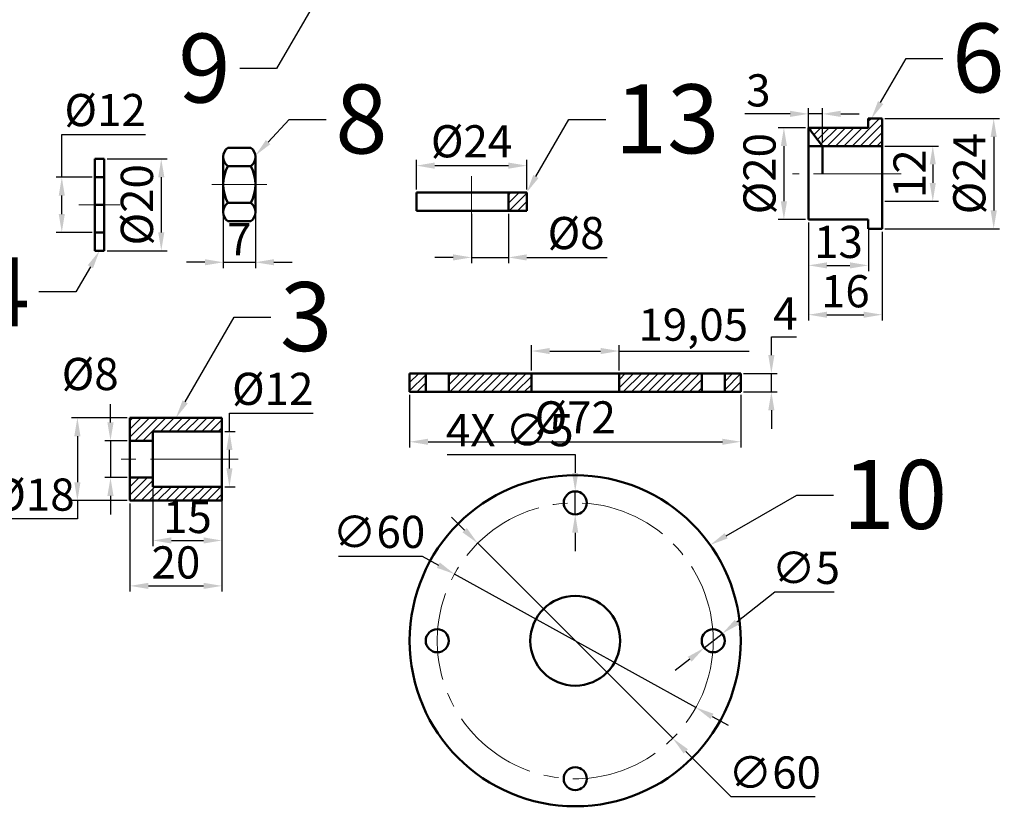
# Model space of a CAD drawing. Units: millimetres. Extents: x 123 to 731, y 468 to 864.
# Tile 3 of 5: x 328 to 542, y 604 to 775. Entities that reach past the tile are written whole.
import ezdxf
from ezdxf import colors
from ezdxf.entities.mleader import LeaderData, LeaderLine
from ezdxf.math import Vec2, Vec3

# ---------------------------------------------------------------- set-up
doc = ezdxf.new("R2010")
doc.units = ezdxf.units.MM
doc.linetypes.add('CENTER2', pattern=[28.575, 19.05, -3.175, 3.175, -3.175])
for name, color, linetype, lineweight in [('M-CNTR', 1, 'CENTER2', 18), ('M-DIMS', 2, 'Continuous', 25), ('M-HATC', 8, 'Continuous', 18), ('M-OUTL', 7, 'Continuous', 50), ('M-TEXT', 3, 'Continuous', 25)]:
    doc.layers.add(name, color=color, linetype=linetype, lineweight=lineweight)
doc.styles.get("Standard").update_dxf_attribs({"font": 'arial.ttf'})
doc.dimstyles.new('ISO-25', dxfattribs={"dimtxt": 7, "dimasz": 4, "dimexe": 1.25, "dimexo": 0.625, "dimtad": 1, "dimtoh": 1, "dimtxsty": 'Standard', "dimcen": 2.5, "dimadec": 0, "dimazin": 0, "dimtfac": 1, "dimtmove": 0, "dimatfit": 3, "dimfxl": 1, "dimarcsym": 0})

# ---------------------------------------------------------------- blocks, each defined once
blk = doc.blocks.new('*D38')
at = {"layer": 'Defpoints', "color": 0, "transparency": 16777216}
for p in [(372.22, 733.55), (379.22, 733.55), (379.22, 722.64)]:
    blk.add_point(p, dxfattribs=at)
at = {"layer": 'M-DIMS', "color": 0, "lineweight": -2, "transparency": 16777216}
for p, q in [((372.22, 732.92), (372.22, 721.39)), ((379.22, 732.92), (379.22, 721.39)), ((368.22, 722.64), (364.22, 722.64)), ((372.22, 722.64), (379.22, 722.64)), ((383.22, 722.64), (387.22, 722.64))]:
    blk.add_line(p, q, dxfattribs=at)
at = {"layer": 'M-DIMS', "color": 0, "transparency": 16777216}
for points in [[(368.22, 723.31), (368.22, 721.98), (372.22, 722.64)], [(383.22, 723.31), (383.22, 721.98), (379.22, 722.64)]]:
    blk.add_solid(points, dxfattribs=at)
at = {"layer": 'M-DIMS', "color": 0, "transparency": 16777216, "insert": (375.72, 726.77), "char_height": 7, "attachment_point": 5}
blk.add_mtext('7', dxfattribs=at)
blk = doc.blocks.new('*U39')
at = {"layer": 'M-CNTR', "color": 0, "transparency": 16777216}
blk.add_line((6, 0), (-6, 0), dxfattribs=at)
blk = doc.blocks.new('*U41')
at = {"layer": 'M-CNTR', "color": 0, "transparency": 16777216}
blk.add_line((4.5, 0), (-4.5, 0), dxfattribs=at)
blk = doc.blocks.new('*D43')
at = {"layer": 'Defpoints', "color": 0, "transparency": 16777216}
for p in [(344.32, 741.14), (337.11, 729.14), (344.32, 729.14)]:
    blk.add_point(p, dxfattribs=at)
at = {"layer": 'M-DIMS', "color": 0, "lineweight": -2, "transparency": 16777216}
for p, q in [((337.11, 741.14), (337.11, 750.44)), ((337.11, 750.44), (355.3, 750.44)), ((343.7, 741.14), (335.86, 741.14)), ((337.11, 733.14), (337.11, 737.14)), ((343.7, 729.14), (335.86, 729.14))]:
    blk.add_line(p, q, dxfattribs=at)
at = {"layer": 'M-DIMS', "color": 0, "transparency": 16777216}
for points in [[(336.44, 737.14), (337.77, 737.14), (337.11, 741.14)], [(336.44, 733.14), (337.77, 733.14), (337.11, 729.14)]]:
    blk.add_solid(points, dxfattribs=at)
at = {"layer": 'M-DIMS', "color": 0, "transparency": 16777216, "insert": (346.52, 754.84), "char_height": 7, "attachment_point": 5}
blk.add_mtext('%%C12', dxfattribs=at)
blk = doc.blocks.new('*D44')
at = {"layer": 'Defpoints', "color": 0, "transparency": 16777216}
for p in [(346.32, 745.14), (346.32, 725.14), (358.74, 725.14)]:
    blk.add_point(p, dxfattribs=at)
at = {"layer": 'M-DIMS', "color": 0, "lineweight": -2, "transparency": 16777216}
for p, q in [((346.95, 745.14), (359.99, 745.14)), ((358.74, 741.14), (358.74, 729.14)), ((346.95, 725.14), (359.99, 725.14))]:
    blk.add_line(p, q, dxfattribs=at)
at = {"layer": 'M-DIMS', "color": 0, "transparency": 16777216}
for points in [[(358.08, 741.14), (359.41, 741.14), (358.74, 745.14)], [(358.08, 729.14), (359.41, 729.14), (358.74, 725.14)]]:
    blk.add_solid(points, dxfattribs=at)
at = {"layer": 'M-DIMS', "color": 0, "transparency": 16777216, "insert": (354.35, 735.14), "char_height": 7, "attachment_point": 5, "rotation": 90}
blk.add_mtext('%%C20', dxfattribs=at)
blk = doc.blocks.new('*U45')
at = {"layer": 'M-CNTR', "color": 0, "transparency": 16777216}
blk.add_line((0, -5.5), (0, 5.5), dxfattribs=at)
blk = doc.blocks.new('*D47')
at = {"layer": 'Defpoints', "color": 0, "transparency": 16777216}
for p in [(438.21, 743.66), (414.21, 737.84), (438.21, 737.84)]:
    blk.add_point(p, dxfattribs=at)
at = {"layer": 'M-DIMS', "color": 0, "lineweight": -2, "transparency": 16777216}
for p, q in [((414.21, 738.46), (414.21, 744.91)), ((418.21, 743.66), (434.21, 743.66)), ((438.21, 738.46), (438.21, 744.91))]:
    blk.add_line(p, q, dxfattribs=at)
at = {"layer": 'M-DIMS', "color": 0, "transparency": 16777216}
for points in [[(418.21, 744.33), (418.21, 742.99), (414.21, 743.66)], [(434.21, 744.33), (434.21, 742.99), (438.21, 743.66)]]:
    blk.add_solid(points, dxfattribs=at)
at = {"layer": 'M-DIMS', "color": 0, "transparency": 16777216, "insert": (426.21, 748.05), "char_height": 7, "attachment_point": 5}
blk.add_mtext('%%C24', dxfattribs=at)
blk = doc.blocks.new('*D48')
at = {"layer": 'Defpoints', "color": 0, "transparency": 16777216}
for p in [(426.21, 733.84), (434.21, 733.84), (434.21, 723.7)]:
    blk.add_point(p, dxfattribs=at)
at = {"layer": 'M-DIMS', "color": 0, "lineweight": -2, "transparency": 16777216}
for p, q in [((426.21, 733.21), (426.21, 722.45)), ((434.21, 733.21), (434.21, 722.45)), ((422.21, 723.7), (418.21, 723.7)), ((426.21, 723.7), (434.21, 723.7)), ((438.21, 723.7), (455.68, 723.7))]:
    blk.add_line(p, q, dxfattribs=at)
at = {"layer": 'M-DIMS', "color": 0, "transparency": 16777216}
for points in [[(422.21, 724.36), (422.21, 723.03), (426.21, 723.7)], [(438.21, 724.36), (438.21, 723.03), (434.21, 723.7)]]:
    blk.add_solid(points, dxfattribs=at)
at = {"layer": 'M-DIMS', "color": 0, "transparency": 16777216, "insert": (448.94, 728.09), "char_height": 7, "attachment_point": 5}
blk.add_mtext('%%C8', dxfattribs=at)
blk = doc.blocks.new('*U54')
at = {"layer": 'M-CNTR', "color": 0, "transparency": 16777216}
blk.add_line((13.65, 0), (-10, 0), dxfattribs=at)
blk = doc.blocks.new('*D55')
at = {"layer": 'Defpoints', "color": 0, "transparency": 16777216}
for p in [(499.49, 751.91), (494.13, 731.91), (499.49, 731.91)]:
    blk.add_point(p, dxfattribs=at)
at = {"layer": 'M-DIMS', "color": 0, "lineweight": -2, "transparency": 16777216}
for p, q in [((498.86, 751.91), (492.88, 751.91)), ((494.13, 747.91), (494.13, 735.91)), ((498.86, 731.91), (492.88, 731.91))]:
    blk.add_line(p, q, dxfattribs=at)
at = {"layer": 'M-DIMS', "color": 0, "transparency": 16777216}
for points in [[(493.46, 747.91), (494.8, 747.91), (494.13, 751.91)], [(493.46, 735.91), (494.8, 735.91), (494.13, 731.91)]]:
    blk.add_solid(points, dxfattribs=at)
at = {"layer": 'M-DIMS', "color": 0, "transparency": 16777216, "insert": (489.73, 741.91), "char_height": 7, "attachment_point": 5, "rotation": 90}
blk.add_mtext('%%C20', dxfattribs=at)
blk = doc.blocks.new('*D56')
at = {"layer": 'Defpoints', "color": 0, "transparency": 16777216}
for p in [(502.49, 754.92), (499.49, 747.91), (502.49, 747.91)]:
    blk.add_point(p, dxfattribs=at)
at = {"layer": 'M-DIMS', "color": 0, "lineweight": -2, "transparency": 16777216}
for p, q in [((499.49, 748.54), (499.49, 756.17)), ((502.49, 748.54), (502.49, 756.17)), ((495.49, 754.92), (485.65, 754.92)), ((502.49, 754.92), (499.49, 754.92)), ((506.49, 754.92), (510.49, 754.92))]:
    blk.add_line(p, q, dxfattribs=at)
at = {"layer": 'M-DIMS', "color": 0, "transparency": 16777216}
for points in [[(495.49, 755.59), (495.49, 754.25), (499.49, 754.92)], [(506.49, 755.59), (506.49, 754.25), (502.49, 754.92)]]:
    blk.add_solid(points, dxfattribs=at)
at = {"layer": 'M-DIMS', "color": 0, "transparency": 16777216, "insert": (488.57, 759.12), "char_height": 7, "attachment_point": 5}
blk.add_mtext('3', dxfattribs=at)
blk = doc.blocks.new('*D57')
at = {"layer": 'Defpoints', "color": 0, "transparency": 16777216}
for p in [(515.49, 747.91), (515.49, 735.91), (526.5, 735.91)]:
    blk.add_point(p, dxfattribs=at)
at = {"layer": 'M-DIMS', "color": 0, "lineweight": -2, "transparency": 16777216}
for p, q in [((516.11, 747.91), (527.75, 747.91)), ((526.5, 743.91), (526.5, 739.91)), ((516.11, 735.91), (527.75, 735.91))]:
    blk.add_line(p, q, dxfattribs=at)
at = {"layer": 'M-DIMS', "color": 0, "transparency": 16777216}
for points in [[(525.83, 743.91), (527.17, 743.91), (526.5, 747.91)], [(525.83, 739.91), (527.17, 739.91), (526.5, 735.91)]]:
    blk.add_solid(points, dxfattribs=at)
at = {"layer": 'M-DIMS', "color": 0, "transparency": 16777216, "insert": (522.36, 741.91), "char_height": 7, "attachment_point": 5, "rotation": 90}
blk.add_mtext('12', dxfattribs=at)
blk = doc.blocks.new('*D58')
at = {"layer": 'Defpoints', "color": 0, "transparency": 16777216}
for p in [(515.49, 753.91), (515.49, 729.91), (539.75, 729.91)]:
    blk.add_point(p, dxfattribs=at)
at = {"layer": 'M-DIMS', "color": 0, "lineweight": -2, "transparency": 16777216}
for p, q in [((516.11, 753.91), (541, 753.91)), ((539.75, 749.91), (539.75, 733.91)), ((516.11, 729.91), (541, 729.91))]:
    blk.add_line(p, q, dxfattribs=at)
at = {"layer": 'M-DIMS', "color": 0, "transparency": 16777216}
for points in [[(539.08, 749.91), (540.42, 749.91), (539.75, 753.91)], [(539.08, 733.91), (540.42, 733.91), (539.75, 729.91)]]:
    blk.add_solid(points, dxfattribs=at)
at = {"layer": 'M-DIMS', "color": 0, "transparency": 16777216, "insert": (535.36, 741.91), "char_height": 7, "attachment_point": 5, "rotation": 90}
blk.add_mtext('%%C24', dxfattribs=at)
blk = doc.blocks.new('*D59')
at = {"layer": 'Defpoints', "color": 0, "transparency": 16777216}
for p in [(499.49, 731.91), (512.49, 731.91), (512.49, 721.97)]:
    blk.add_point(p, dxfattribs=at)
at = {"layer": 'M-DIMS', "color": 0, "lineweight": -2, "transparency": 16777216}
for p, q in [((499.49, 731.29), (499.49, 720.72)), ((512.49, 731.29), (512.49, 720.72)), ((503.49, 721.97), (508.49, 721.97))]:
    blk.add_line(p, q, dxfattribs=at)
at = {"layer": 'M-DIMS', "color": 0, "transparency": 16777216}
for points in [[(503.49, 722.63), (503.49, 721.3), (499.49, 721.97)], [(508.49, 722.63), (508.49, 721.3), (512.49, 721.97)]]:
    blk.add_solid(points, dxfattribs=at)
at = {"layer": 'M-DIMS', "color": 0, "transparency": 16777216, "insert": (505.99, 726.17), "char_height": 7, "attachment_point": 5}
blk.add_mtext('13', dxfattribs=at)
blk = doc.blocks.new('*D60')
at = {"layer": 'Defpoints', "color": 0, "transparency": 16777216}
for p in [(499.49, 731.91), (515.49, 729.91), (515.49, 711.24)]:
    blk.add_point(p, dxfattribs=at)
at = {"layer": 'M-DIMS', "color": 0, "lineweight": -2, "transparency": 16777216}
for p, q in [((499.49, 731.29), (499.49, 709.99)), ((515.49, 729.29), (515.49, 709.99)), ((503.49, 711.24), (511.49, 711.24))]:
    blk.add_line(p, q, dxfattribs=at)
at = {"layer": 'M-DIMS', "color": 0, "transparency": 16777216}
for points in [[(503.49, 711.9), (503.49, 710.57), (499.49, 711.24)], [(511.49, 711.9), (511.49, 710.57), (515.49, 711.24)]]:
    blk.add_solid(points, dxfattribs=at)
at = {"layer": 'M-DIMS', "color": 0, "transparency": 16777216, "insert": (507.49, 715.44), "char_height": 7, "attachment_point": 5}
blk.add_mtext('16', dxfattribs=at)
blk = doc.blocks.new('*U70')
at = {"layer": 'M-CNTR', "color": 0, "transparency": 16777216}
blk.add_line((13.5, 0), (-13.5, 0), dxfattribs=at)
blk = doc.blocks.new('*D72')
at = {"layer": 'Defpoints', "color": 0, "transparency": 16777216}
for p in [(351.93, 683.82), (347.7, 675.82), (351.93, 675.82)]:
    blk.add_point(p, dxfattribs=at)
at = {"layer": 'M-DIMS', "color": 0, "lineweight": -2, "transparency": 16777216}
for p, q in [((347.7, 687.82), (347.7, 691.82)), ((351.31, 683.82), (346.45, 683.82)), ((347.7, 683.82), (347.7, 675.82)), ((351.31, 675.82), (346.45, 675.82)), ((347.7, 671.82), (347.7, 667.82))]:
    blk.add_line(p, q, dxfattribs=at)
at = {"layer": 'M-DIMS', "color": 0, "transparency": 16777216}
for points in [[(347.03, 687.82), (348.37, 687.82), (347.7, 683.82)], [(347.03, 671.82), (348.37, 671.82), (347.7, 675.82)]]:
    blk.add_solid(points, dxfattribs=at)
at = {"layer": 'M-DIMS', "color": 0, "transparency": 16777216, "insert": (343.28, 697.44), "char_height": 7, "attachment_point": 5}
blk.add_mtext('%%C8', dxfattribs=at)
blk = doc.blocks.new('*D73')
at = {"layer": 'Defpoints', "color": 0, "transparency": 16777216}
for p in [(351.93, 688.82), (340.5, 670.82), (351.93, 670.82)]:
    blk.add_point(p, dxfattribs=at)
at = {"layer": 'M-DIMS', "color": 0, "lineweight": -2, "transparency": 16777216}
for p, q in [((351.31, 688.82), (339.25, 688.82)), ((340.5, 684.82), (340.5, 674.82)), ((351.31, 670.82), (339.25, 670.82)), ((340.5, 670.82), (340.5, 666.82)), ((340.5, 666.82), (322.22, 666.82))]:
    blk.add_line(p, q, dxfattribs=at)
at = {"layer": 'M-DIMS', "color": 0, "transparency": 16777216}
for points in [[(339.83, 684.82), (341.17, 684.82), (340.5, 688.82)], [(339.83, 674.82), (341.17, 674.82), (340.5, 670.82)]]:
    blk.add_solid(points, dxfattribs=at)
at = {"layer": 'M-DIMS', "color": 0, "transparency": 16777216, "insert": (331.05, 671.21), "char_height": 7, "attachment_point": 5}
blk.add_mtext('%%C18', dxfattribs=at)
blk = doc.blocks.new('*D74')
at = {"layer": 'Defpoints', "color": 0, "transparency": 16777216}
for p in [(356.93, 673.82), (371.93, 673.82), (371.93, 662.14)]:
    blk.add_point(p, dxfattribs=at)
at = {"layer": 'M-DIMS', "color": 0, "lineweight": -2, "transparency": 16777216}
for p, q in [((356.93, 673.19), (356.93, 660.89)), ((371.93, 673.19), (371.93, 660.89)), ((360.93, 662.14), (367.93, 662.14))]:
    blk.add_line(p, q, dxfattribs=at)
at = {"layer": 'M-DIMS', "color": 0, "transparency": 16777216}
for points in [[(360.93, 662.81), (360.93, 661.48), (356.93, 662.14)], [(367.93, 662.81), (367.93, 661.48), (371.93, 662.14)]]:
    blk.add_solid(points, dxfattribs=at)
at = {"layer": 'M-DIMS', "color": 0, "transparency": 16777216, "insert": (364.43, 666.34), "char_height": 7, "attachment_point": 5}
blk.add_mtext('15', dxfattribs=at)
blk = doc.blocks.new('*D75')
at = {"layer": 'Defpoints', "color": 0, "transparency": 16777216}
for p in [(351.93, 670.82), (371.93, 670.82), (371.93, 652.26)]:
    blk.add_point(p, dxfattribs=at)
at = {"layer": 'M-DIMS', "color": 0, "lineweight": -2, "transparency": 16777216}
for p, q in [((351.93, 670.19), (351.93, 651.01)), ((371.93, 670.19), (371.93, 651.01)), ((355.93, 652.26), (367.93, 652.26))]:
    blk.add_line(p, q, dxfattribs=at)
at = {"layer": 'M-DIMS', "color": 0, "transparency": 16777216}
for points in [[(355.93, 652.93), (355.93, 651.6), (351.93, 652.26)], [(367.93, 652.93), (367.93, 651.6), (371.93, 652.26)]]:
    blk.add_solid(points, dxfattribs=at)
at = {"layer": 'M-DIMS', "color": 0, "transparency": 16777216, "insert": (361.93, 656.46), "char_height": 7, "attachment_point": 5}
blk.add_mtext('20', dxfattribs=at)
blk = doc.blocks.new('*D76')
at = {"layer": 'Defpoints', "color": 0, "transparency": 16777216}
for p in [(371.93, 685.82), (371.93, 673.82), (373.56, 673.82)]:
    blk.add_point(p, dxfattribs=at)
at = {"layer": 'M-DIMS', "color": 0, "lineweight": -2, "transparency": 16777216}
for p, q in [((373.56, 685.82), (373.56, 689.82)), ((373.56, 689.82), (391.76, 689.82)), ((372.56, 685.82), (374.81, 685.82)), ((373.56, 677.82), (373.56, 681.82)), ((372.56, 673.82), (374.81, 673.82))]:
    blk.add_line(p, q, dxfattribs=at)
at = {"layer": 'M-DIMS', "color": 0, "transparency": 16777216}
for points in [[(372.9, 681.82), (374.23, 681.82), (373.56, 685.82)], [(372.9, 677.82), (374.23, 677.82), (373.56, 673.82)]]:
    blk.add_solid(points, dxfattribs=at)
at = {"layer": 'M-DIMS', "color": 0, "transparency": 16777216, "insert": (382.97, 694.21), "char_height": 7, "attachment_point": 5}
blk.add_mtext('%%C12', dxfattribs=at)
blk = doc.blocks.new('*D77')
at = {"layer": 'Defpoints', "color": 0, "transparency": 16777216}
for p in [(412.75, 694.45), (484.75, 694.45), (484.75, 683.61)]:
    blk.add_point(p, dxfattribs=at)
at = {"layer": 'M-DIMS', "color": 0, "lineweight": -2, "transparency": 16777216}
for p, q in [((412.75, 693.83), (412.75, 682.36)), ((484.75, 693.83), (484.75, 682.36)), ((416.75, 683.61), (480.75, 683.61))]:
    blk.add_line(p, q, dxfattribs=at)
at = {"layer": 'M-DIMS', "color": 0, "transparency": 16777216}
for points in [[(416.75, 684.27), (416.75, 682.94), (412.75, 683.61)], [(480.75, 684.27), (480.75, 682.94), (484.75, 683.61)]]:
    blk.add_solid(points, dxfattribs=at)
at = {"layer": 'M-DIMS', "color": 0, "transparency": 16777216, "insert": (448.75, 688), "char_height": 7, "attachment_point": 5}
blk.add_mtext('%%C72', dxfattribs=at)
blk = doc.blocks.new('*D78')
at = {"layer": 'Defpoints', "color": 0, "transparency": 16777216}
for p in [(458.28, 703.34), (439.23, 698.45), (458.28, 698.45)]:
    blk.add_point(p, dxfattribs=at)
at = {"layer": 'M-DIMS', "color": 0, "lineweight": -2, "transparency": 16777216}
for p, q in [((439.23, 699.08), (439.23, 704.59)), ((458.28, 699.08), (458.28, 704.59)), ((443.23, 703.34), (454.28, 703.34)), ((458.28, 703.34), (486.54, 703.34))]:
    blk.add_line(p, q, dxfattribs=at)
at = {"layer": 'M-DIMS', "color": 0, "transparency": 16777216}
for points in [[(443.23, 704.01), (443.23, 702.67), (439.23, 703.34)], [(454.28, 704.01), (454.28, 702.67), (458.28, 703.34)]]:
    blk.add_solid(points, dxfattribs=at)
at = {"layer": 'M-DIMS', "color": 0, "transparency": 16777216, "insert": (474.41, 708.17), "char_height": 7, "attachment_point": 5}
blk.add_mtext('19,05', dxfattribs=at)
blk = doc.blocks.new('*D79')
at = {"layer": 'Defpoints', "color": 0, "transparency": 16777216}
for p in [(480.71, 641.87), (476.79, 638.78)]:
    blk.add_point(p, dxfattribs=at)
at = {"layer": 'M-DIMS', "color": 0, "lineweight": -2, "transparency": 16777216}
for p, q in [((492.15, 650.88), (483.86, 644.35)), ((505.03, 650.88), (492.15, 650.88)), ((476.79, 638.78), (480.71, 641.87)), ((473.65, 636.3), (470.5, 633.83))]:
    blk.add_line(p, q, dxfattribs=at)
at = {"layer": 'M-DIMS', "color": 0, "transparency": 16777216}
for points in [[(483.44, 644.87), (484.27, 643.82), (480.71, 641.87)], [(473.23, 636.83), (474.06, 635.78), (476.79, 638.78)]]:
    blk.add_solid(points, dxfattribs=at)
at = {"layer": 'M-DIMS', "color": 0, "transparency": 16777216, "insert": (498.9, 655.27), "char_height": 7, "attachment_point": 5}
blk.add_mtext('∅5', dxfattribs=at)
blk = doc.blocks.new('*D80')
at = {"layer": 'Defpoints', "color": 0, "transparency": 16777216}
for p in [(422.49, 654.83), (475.01, 625.81)]:
    blk.add_point(p, dxfattribs=at)
at = {"layer": 'M-DIMS', "color": 0, "lineweight": -2, "transparency": 16777216}
for p, q in [((397.25, 658.7), (415.49, 658.7)), ((415.49, 658.7), (418.99, 656.77)), ((475.01, 625.81), (422.49, 654.83)), ((478.51, 623.88), (482.01, 621.95))]:
    blk.add_line(p, q, dxfattribs=at)
at = {"layer": 'M-DIMS', "color": 0, "transparency": 16777216}
for points in [[(419.31, 657.35), (418.67, 656.19), (422.49, 654.83)], [(478.83, 624.46), (478.19, 623.3), (475.01, 625.81)]]:
    blk.add_solid(points, dxfattribs=at)
at = {"layer": 'M-DIMS', "color": 0, "transparency": 16777216, "insert": (406.06, 663.1), "char_height": 7, "attachment_point": 5}
blk.add_mtext('∅60', dxfattribs=at)
blk = doc.blocks.new('HEX-NUT')
for p, q in [((6.02, 16), (1.02, 16)), ((1.02, 12), (6.02, 12)), ((1.02, 4), (6.02, 4)), ((1.02, 0), (6.02, 0))]:
    blk.add_line(p, q)
for centre, radius, start, end in [((2.47, 14), 2.47, 125.9888, 234.0112), ((4.57, 14), 2.47, 305.9888, 54.0112), ((8.52, 8), 8.5, 151.9275, 208.0725), ((-1.48, 8), 8.5, 331.9275, 28.0725), ((2.52, 2), 2.5, 126.8697, 233.1303), ((4.52, 2), 2.5, 306.8697, 53.1303)]:
    blk.add_arc(centre, radius, start, end)
blk = doc.blocks.new('*D94')
at = {"layer": 'Defpoints', "color": 0, "transparency": 16777216}
for p in [(484.75, 698.45), (491.4, 698.45), (484.75, 694.45)]:
    blk.add_point(p, dxfattribs=at)
at = {"layer": 'M-DIMS', "color": 0, "lineweight": -2, "transparency": 16777216}
for p, q in [((491.4, 702.45), (491.4, 706.45)), ((491.4, 706.45), (496.87, 706.45)), ((485.38, 698.45), (492.65, 698.45)), ((491.4, 694.45), (491.4, 698.45)), ((485.38, 694.45), (492.65, 694.45)), ((491.4, 690.45), (491.4, 686.45))]:
    blk.add_line(p, q, dxfattribs=at)
at = {"layer": 'M-DIMS', "color": 0, "transparency": 16777216}
for points in [[(490.73, 702.45), (492.07, 702.45), (491.4, 698.45)], [(490.73, 690.45), (492.07, 690.45), (491.4, 694.45)]]:
    blk.add_solid(points, dxfattribs=at)
at = {"layer": 'M-DIMS', "color": 0, "transparency": 16777216, "insert": (494.45, 710.58), "char_height": 7, "attachment_point": 5}
blk.add_mtext('4', dxfattribs=at)
blk = doc.blocks.new('*D96')
at = {"layer": 'Defpoints', "color": 0, "transparency": 16777216}
for p in [(427.54, 661.54), (469.96, 619.11)]:
    blk.add_point(p, dxfattribs=at)
at = {"layer": 'M-DIMS', "color": 0, "lineweight": -2, "transparency": 16777216}
for p, q in [((424.71, 664.37), (421.88, 667.2)), ((427.54, 661.54), (469.96, 619.11)), ((482.69, 606.38), (472.79, 616.28)), ((500.93, 606.38), (482.69, 606.38))]:
    blk.add_line(p, q, dxfattribs=at)
at = {"layer": 'M-DIMS', "color": 0, "transparency": 16777216}
for points in [[(425.18, 664.84), (424.24, 663.9), (427.54, 661.54)], [(473.26, 616.75), (472.32, 615.81), (469.96, 619.11)]]:
    blk.add_solid(points, dxfattribs=at)
at = {"layer": 'M-DIMS', "color": 0, "transparency": 16777216, "insert": (492.12, 610.77), "char_height": 7, "attachment_point": 5}
blk.add_mtext('∅60', dxfattribs=at)
blk = doc.blocks.new('*D97')
at = {"layer": 'Defpoints', "color": 0, "transparency": 16777216}
for p in [(448.75, 672.82), (448.75, 667.82)]:
    blk.add_point(p, dxfattribs=at)
at = {"layer": 'M-DIMS', "color": 0, "lineweight": -2, "transparency": 16777216}
for p, q in [((420.91, 680.82), (448.75, 680.82)), ((448.75, 680.82), (448.75, 676.82)), ((448.75, 667.82), (448.75, 672.82)), ((448.75, 663.82), (448.76, 659.82))]:
    blk.add_line(p, q, dxfattribs=at)
at = {"layer": 'M-DIMS', "color": 0, "transparency": 16777216}
for points in [[(449.41, 676.83), (448.08, 676.82), (448.75, 672.82)], [(449.42, 663.83), (448.09, 663.82), (448.75, 667.82)]]:
    blk.add_solid(points, dxfattribs=at)
at = {"layer": 'M-DIMS', "color": 0, "transparency": 16777216, "insert": (434.52, 685.22), "char_height": 7, "attachment_point": 5}
blk.add_mtext('4X ∅5', dxfattribs=at)

msp = doc.modelspace()

# ---------------------------------------------------------------- hatches: boundary and pattern name
at = {"layer": 'M-HATC'}
h = msp.add_hatch(dxfattribs=at)
h.set_pattern_fill('ANSI31', color=256, scale=0.4)
h.set_pattern_definition([(45, (-32.4287, 0), (-0.8980256, 0.8980256), [])])
h.paths.add_polyline_path([(499.4872, 751.9133), (502.4872, 747.9133), (515.4872, 747.9133), (515.4872, 753.9133), (512.4872, 753.9133), (512.4872, 751.9133)])
h = msp.add_hatch(dxfattribs=at)
h.set_pattern_fill('ANSI31', color=256, scale=0.4)
h.set_pattern_definition([(45, (-30.5264, 6.709), (-0.8980256, 0.8980256), [])])
h.paths.add_polyline_path([(434.2097, 733.837), (438.2097, 733.837), (438.2097, 737.837), (434.2097, 737.837)])
h = msp.add_hatch(dxfattribs=at)
h.set_pattern_fill('ANSI31', color=256, scale=0.4)
h.set_pattern_definition([(45, (-31.5995, 122.8167), (-0.8980256, 0.8980256), [])])
h.paths.add_polyline_path([(416.251, 698.4517), (412.751, 698.4517), (412.751, 694.4517), (416.251, 694.4517)])
h.paths.add_polyline_path([(439.226, 694.4517), (439.226, 698.4517), (421.251, 698.4517), (421.251, 694.4517)])
h.paths.add_polyline_path([(476.251, 694.4517), (476.251, 698.4517), (458.276, 698.4517), (458.276, 694.4517)])
h.paths.add_polyline_path([(481.251, 694.4517), (484.751, 694.4517), (484.751, 698.4517), (481.251, 698.4517)])
h = msp.add_hatch(dxfattribs=at)
h.set_pattern_fill('ANSI31', color=256, scale=0.4)
h.set_pattern_definition([(45, (-13.901, 8.0257), (-0.8980256, 0.8980256), [])])
h.paths.add_polyline_path([(351.9314, 683.8159), (356.9314, 683.8159), (356.9314, 685.8159), (371.9314, 685.8159), (371.9314, 688.8159), (351.9314, 688.8159)])
h.paths.add_polyline_path([(371.9314, 670.8159), (371.9314, 673.8159), (356.9314, 673.8159), (356.9314, 675.8159), (351.9314, 675.8159), (351.9314, 670.8159)])

# ---------------------------------------------------------------- linework, layer by layer
at = {"layer": 'M-CNTR'}
msp.add_circle((448.751, 640.3248), 30, dxfattribs=at)
at = {"layer": 'M-OUTL'}
for p, q in [((515.4872, 753.9133), (512.4872, 753.9133)), ((512.4872, 753.9133), (512.4872, 751.9133)), ((515.4872, 729.9133), (515.4872, 753.9133)), ((499.4872, 751.9133), (499.4872, 731.9133)), ((512.4872, 751.9133), (499.4872, 751.9133)), ((502.4872, 747.9133), (499.4872, 751.9133)), ((499.4872, 747.9133), (502.4872, 747.9133)), ((502.4872, 747.9133), (502.4872, 741.9133)), ((502.4872, 747.9133), (515.4872, 747.9133)), ((344.3205, 745.1393), (344.3205, 725.1393)), ((346.3205, 745.1393), (344.3205, 745.1393)), ((346.3205, 725.1393), (346.3205, 745.1393)), ((372.2169, 745.8609), (372.2169, 733.5485)), ((379.2169, 733.5485), (379.2169, 745.8609)), ((344.3205, 741.1393), (346.3205, 741.1393)), ((438.2097, 737.837), (414.2097, 737.837)), ((414.2097, 737.837), (414.2097, 733.837)), ((434.2097, 737.837), (434.2097, 733.837)), ((438.2097, 733.837), (438.2097, 737.837)), ((344.3205, 735.1393), (346.3205, 735.1393)), ((414.2097, 733.837), (438.2097, 733.837)), ((499.4872, 731.9133), (512.4872, 731.9133)), ((512.4872, 731.9133), (512.4872, 729.9133)), ((344.3205, 729.1393), (346.3205, 729.1393)), ((512.4872, 729.9133), (515.4872, 729.9133)), ((344.3205, 725.1393), (346.3205, 725.1393)), ((484.751, 698.4517), (412.751, 698.4517)), ((412.751, 698.4517), (412.751, 694.4517)), ((416.251, 694.4517), (416.251, 698.4517)), ((421.251, 694.4517), (421.251, 698.4517)), ((439.226, 698.4517), (439.226, 694.4517)), ((458.276, 698.4517), (458.276, 694.4517)), ((476.251, 694.4517), (476.251, 698.4517)), ((481.251, 694.4517), (481.251, 698.4517)), ((484.751, 694.4517), (484.751, 698.4517)), ((412.751, 694.4517), (484.751, 694.4517)), ((351.9314, 688.8159), (351.9314, 670.8159)), ((371.9314, 688.8159), (351.9314, 688.8159)), ((371.9314, 670.8159), (371.9314, 688.8159)), ((371.9314, 685.8159), (356.9314, 685.8159)), ((356.9314, 685.8159), (356.9314, 673.8159)), ((351.9314, 683.8159), (356.9314, 683.8159)), ((351.9314, 675.8159), (356.9314, 675.8159)), ((356.9314, 673.8159), (371.9314, 673.8159)), ((351.9314, 670.8159), (371.9314, 670.8159))]:
    msp.add_line(p, q, dxfattribs=at)
for centre, radius in [((448.751, 640.3248), 36), ((448.751, 670.3248), 2.5), ((448.751, 640.3248), 9.7625), ((418.751, 640.3248), 2.5), ((478.751, 640.3248), 2.5), ((448.751, 610.3248), 2.5)]:
    msp.add_circle(centre, radius, dxfattribs=at)

# ---------------------------------------------------------------- block references
at = {"layer": 'M-CNTR'}
for name, p in [('*U45', (426.2097, 735.837)), ('*U54', (505.9872, 741.9133)), ('*U39', (375.7169, 739.5526)), ('*U41', (345.3205, 735.1393)), ('*U70', (361.9314, 679.8159))]:
    msp.add_blockref(name, p, dxfattribs=at)
at = {"layer": 'M-OUTL'}
msp.add_blockref('HEX-NUT', (372.198, 731.553), dxfattribs=at)

# ---------------------------------------------------------------- dimensions: what is measured, and where the dimension line sits
at = {"layer": 'M-DIMS'}
dim = msp.add_linear_dim(base=(502.4872, 754.9192), p1=(499.4872, 747.9133), p2=(502.4872, 747.9133), dimstyle='ISO-25', override={"dimclrd": 0, "dimclre": 0, "dimclrt": 0}, dxfattribs=at)
dim.commit()
dim.dimension.update_dxf_attribs({"geometry": '*D56', "text_midpoint": (488.5702, 754.9192), "dimtype": 160})
for base, p1, p2, override, picture, middle in [((337.1058, 729.1393), (344.3205, 741.1393), (344.3205, 729.1393), {"dimclrd": 0, "dimclre": 0, "dimclrt": 0}, '*D43', (346.5166, 750.4444)), ((347.7005, 675.8159), (351.9314, 683.8159), (351.9314, 675.8159), {"dimclrd": 0, "dimclre": 0, "dimclrt": 0, "dimtmove": 2}, '*D72', (343.2759, 697.4433)), ((373.5627, 673.8159), (371.9314, 685.8159), (371.9314, 673.8159), {"dimclrd": 0, "dimclre": 0, "dimclrt": 0}, '*D76', (382.9736, 689.8159))]:
    dim = msp.add_linear_dim(base=base, p1=p1, p2=p2, angle=90, text='%%C<>', dimstyle='ISO-25', override=override, dxfattribs=at)
    dim.commit()
    dim.dimension.update_dxf_attribs({"geometry": picture, "text_midpoint": middle, "dimtype": 160})
for base, p1, p2, picture, middle in [((539.7502, 729.9133), (515.4872, 753.9133), (515.4872, 729.9133), '*D58', (535.3555, 741.9133)), ((494.1283, 731.9133), (499.4872, 751.9133), (499.4872, 731.9133), '*D55', (489.7336, 741.9133)), ((358.7435, 725.1393), (346.3205, 745.1393), (346.3205, 725.1393), '*D44', (354.3487, 735.1393)), ((340.5007, 670.8159), (351.9314, 688.8159), (351.9314, 670.8159), '*D73', (331.0469, 671.2107))]:
    dim = msp.add_linear_dim(base=base, p1=p1, p2=p2, angle=90, text='%%C<>', dimstyle='ISO-25', override={"dimclrd": 0, "dimclre": 0, "dimclrt": 0}, dxfattribs=at)
    dim.commit()
    dim.dimension.update_dxf_attribs({"geometry": picture, "text_midpoint": middle})
for base, p1, p2, picture, middle in [((438.2097, 743.6593), (414.2097, 737.837), (438.2097, 737.837), '*D47', (426.2097, 748.0541)), ((434.2097, 723.6956), (426.2097, 733.837), (434.2097, 733.837), '*D48', (448.9442, 728.0903)), ((484.751, 683.6051), (412.751, 694.4517), (484.751, 694.4517), '*D77', (448.751, 687.9999))]:
    dim = msp.add_linear_dim(base=base, p1=p1, p2=p2, text='%%C<>', dimstyle='ISO-25', override={"dimclrd": 0, "dimclre": 0, "dimclrt": 0}, dxfattribs=at)
    dim.commit()
    dim.dimension.update_dxf_attribs({"geometry": picture, "text_midpoint": middle})
for base, p1, p2, override, picture, middle in [((526.5016, 735.9133), (515.4872, 747.9133), (515.4872, 735.9133), {"dimclrd": 0, "dimclre": 0, "dimclrt": 0}, '*D57', (522.3623, 741.9133)), ((491.401, 698.4517), (484.751, 694.4517), (484.751, 698.4517), {"dimdec": 0, "dimlfac": 1, "dimrnd": 0, "dimzin": 0, "dimdsep": 46, "dimlunit": 2}, '*D94', (494.4469, 710.5767))]:
    dim = msp.add_linear_dim(base=base, p1=p1, p2=p2, angle=90, dimstyle='ISO-25', override=override, dxfattribs=at)
    dim.commit()
    dim.dimension.update_dxf_attribs({"geometry": picture, "text_midpoint": middle})
for base, p1, p2, picture, middle in [((379.2169, 722.6433), (372.2169, 733.5485), (379.2169, 733.5485), '*D38', (375.7169, 726.7683)), ((512.4872, 721.9654), (499.4872, 731.9133), (512.4872, 731.9133), '*D59', (505.9872, 726.1668)), ((515.4872, 711.2382), (499.4872, 731.9133), (515.4872, 729.9133), '*D60', (507.4872, 715.4372)), ((458.276, 703.3383), (439.226, 698.4517), (458.276, 698.4517), '*D78', (474.4085, 708.17)), ((371.9314, 662.1442), (356.9314, 673.8159), (371.9314, 673.8159), '*D74', (364.4314, 666.3432)), ((371.9314, 652.2619), (351.9314, 670.8159), (371.9314, 670.8159), '*D75', (361.9314, 656.4609))]:
    dim = msp.add_linear_dim(base=base, p1=p1, p2=p2, dimstyle='ISO-25', override={"dimclrd": 0, "dimclre": 0, "dimclrt": 0}, dxfattribs=at)
    dim.commit()
    dim.dimension.update_dxf_attribs({"geometry": picture, "text_midpoint": middle})
dim = msp.add_diameter_dim_2p(p1=(448.7521, 667.8248), p2=(448.75, 672.8248), text='4X <>', dimstyle='ISO-25', override={"dimdec": 0, "dimlfac": 1, "dimrnd": 0, "dimzin": 0, "dimdsep": 46, "dimlunit": 2}, dxfattribs=at)
dim.commit()
dim.dimension.update_dxf_attribs({"geometry": '*D97', "text_midpoint": (434.5179, 680.8248), "dimtype": 163})
dim = msp.add_diameter_dim_2p(p1=(475.0087, 625.8149), p2=(422.4934, 654.8348), dimstyle='ISO-25', override={"dimclrd": 0, "dimclre": 0, "dimclrt": 0}, dxfattribs=at)
dim.commit()
dim.dimension.update_dxf_attribs({"geometry": '*D80', "text_midpoint": (406.0567, 663.0988)})
for p1, p2, override, picture, middle in [((427.5408, 661.541), (469.9613, 619.1087), {"dimdec": 0, "dimlfac": 1, "dimrnd": 0, "dimzin": 0, "dimdsep": 46, "dimlunit": 2}, '*D96', (492.1221, 606.379)), ((476.7873, 638.7777), (480.7148, 641.872), {"dimclrd": 0, "dimclre": 0, "dimclrt": 0}, '*D79', (498.9017, 650.8795))]:
    dim = msp.add_diameter_dim_2p(p1=p1, p2=p2, dimstyle='ISO-25', override=override, dxfattribs=at)
    dim.commit()
    dim.dimension.update_dxf_attribs({"geometry": picture, "text_midpoint": middle, "dimtype": 163})

# ---------------------------------------------------------------- leaders
at = {"layer": 'M-TEXT'}
ml = msp.add_multileader_mtext('Standard', dxfattribs=at)
ml.set_content('9', color=256)
ml.set_leader_properties()
ml.build(insert=Vec2(0, 0))
ctx = ml.context
ctx.base_point, ctx.char_height, ctx.plane_origin = Vec3(361.9336, 764.7505), 15, Vec3(396.0835, 786.0311)
ctx.text_align_type = 2
notes = []
notes.append((ctx, [(0, (1, 1, 0), (383.7971, 764.7505), (-1, 0), 8, [(0, [(396.0835, 786.0311)], 0, [])])]))
ctx.mtext.insert, ctx.mtext.alignment, ctx.mtext.flow_direction = Vec3(373.7971, 772.3784), 3, 5
ml = msp.add_multileader_mtext('Standard', dxfattribs=at)
ml.set_content('6', color=256)
ml.set_leader_properties()
ml.build(insert=Vec2(0, 0))
ctx = ml.context
ctx.base_point, ctx.char_height, ctx.plane_origin = Vec3(528.6981, 766.9623), 15, Vec3(513.1642, 753.9133)
notes.append((ctx, [(0, (1, 1, 0), (520.6981, 766.9623), (1, 0), 8, [(0, [(513.1642, 753.9133)], 0, [])])]))
ctx.mtext.insert, ctx.mtext.flow_direction = Vec3(530.6981, 774.5902), 5
ml = msp.add_multileader_mtext('Standard', dxfattribs=at)
ml.set_content('8', color=256)
ml.set_leader_properties()
ml.build(insert=Vec2(0, 0))
ctx = ml.context
ctx.base_point, ctx.char_height, ctx.plane_origin = Vec3(394.5781, 753.6778), 15, Vec3(379.2169, 745.8609)
notes.append((ctx, [(0, (1, 1, 0), (386.5781, 753.6778), (1, 0), 8, [(0, [(379.2169, 745.8609)], 0, [])])]))
ctx.mtext.insert, ctx.mtext.flow_direction = Vec3(396.5781, 761.3057), 5
ml = msp.add_multileader_mtext('Standard', dxfattribs=at)
ml.set_content('13', color=256)
ml.set_leader_properties()
ml.build(insert=Vec2(0, 0))
ctx = ml.context
ctx.base_point, ctx.char_height, ctx.plane_origin = Vec3(455.3744, 753.7106), 15, Vec3(438.2097, 737.837)
notes.append((ctx, [(0, (1, 1, 0), (447.3744, 753.7106), (1, 0), 8, [(0, [(438.2097, 737.837)], 0, [])])]))
ctx.mtext.insert, ctx.mtext.flow_direction = Vec3(457.3744, 761.3437), 5
ml = msp.add_multileader_mtext('Standard', dxfattribs=at)
ml.set_content('4', color=256)
ml.set_leader_properties()
ml.build(insert=Vec2(0, 0))
ctx = ml.context
ctx.base_point, ctx.char_height, ctx.plane_origin = Vec3(317.7754, 716.1847), 15, Vec3(345.3205, 725.1393)
ctx.text_align_type = 2
notes.append((ctx, [(0, (1, 1, 0), (340.1506, 716.1847), (-1, 0), 8, [(0, [(345.3205, 725.1393)], 0, [])])]))
ctx.mtext.insert, ctx.mtext.alignment, ctx.mtext.flow_direction = Vec3(330.1506, 723.6847), 3, 5
ml = msp.add_multileader_mtext('Standard', dxfattribs=at)
ml.set_content('3', color=256)
ml.set_leader_properties()
ml.build(insert=Vec2(0, 0))
ctx = ml.context
ctx.base_point, ctx.char_height, ctx.plane_origin = Vec3(382.5657, 710.6992), 15, Vec3(361.9314, 688.8159)
notes.append((ctx, [(0, (1, 1, 0), (374.5657, 710.6992), (1, 0), 8, [(0, [(361.9314, 688.8159)], 0, [])])]))
ctx.mtext.insert, ctx.mtext.flow_direction = Vec3(384.5657, 718.3322), 5
ml = msp.add_multileader_mtext('Standard', dxfattribs=at)
ml.set_content('10', color=256)
ml.set_leader_properties()
ml.build(insert=Vec2(0, 0))
ctx = ml.context
ctx.base_point, ctx.char_height, ctx.plane_origin = Vec3(504.9102, 672.0192), 15, Vec3(478.1069, 661.1631)
notes.append((ctx, [(0, (1, 1, 0), (496.9102, 672.0192), (1, 0), 8, [(0, [(478.1069, 661.1631)], 0, [])])]))
ctx.mtext.insert, ctx.mtext.flow_direction = Vec3(506.9102, 679.6471), 5
for ctx, leaders in notes:
    for number, flags, end, landing, length, lines in leaders:
        leader = LeaderData()
        leader.index, (leader.has_last_leader_line, leader.has_dogleg_vector, leader.attachment_direction) = number, flags
        leader.last_leader_point, leader.dogleg_vector, leader.dogleg_length = Vec3(end), Vec3(landing), length
        for number, points, colour, breaks in lines:
            line = LeaderLine()
            line.index, line.vertices, line.color, line.breaks = number, Vec3.list(points), colors.encode_raw_color(colour), breaks
            leader.lines.append(line)
        ctx.leaders.append(leader)

doc.saveas('drawing.dxf')
